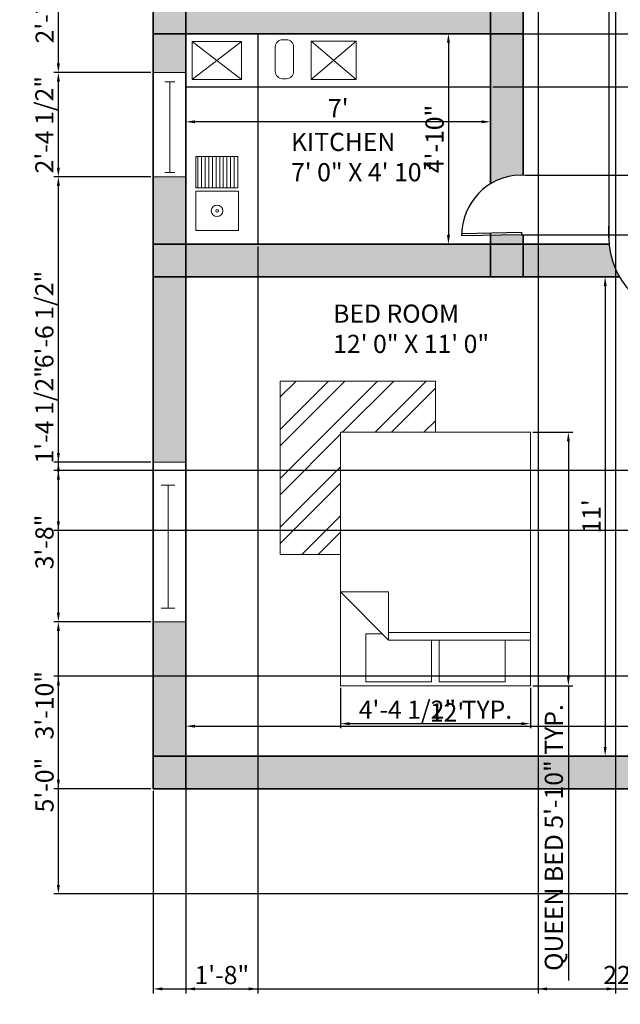
# Model space of a CAD drawing. Units: millimetres. Extents: x 2803 to 3393, y 965 to 1464.
# Tile 1 of 6: x 2803 to 2968, y 965 to 1236. Entities that reach past the tile are written whole.
import ezdxf

# ---------------------------------------------------------------- set-up
doc = ezdxf.new("R2010")
doc.units = ezdxf.units.MM
for name, color, linetype, lineweight in [('A-ANNO-DIMS', 150, 'Continuous', 18), ('A-AREA-IDEN', 200, 'Continuous', 25), ('A-FLOR-CASE', 70, 'Continuous', 25), ('A-FLOR-FIXT', 70, 'Continuous', 18), ('A-FLOR-FIXT-PATT', 70, 'Continuous', 13), ('A-FLOR-PATT', 3, 'Continuous', 13), ('A-WALL-PATT', 2, 'Continuous', 13), ('doors', 10, 'Continuous', 25), ('furniture', 70, 'Continuous', 18), ('walls', 2, 'Continuous', 35), ('windows', 30, 'Continuous', 20)]:
    doc.layers.add(name, color=color, linetype=linetype, lineweight=lineweight)
doc.styles.get("Standard").update_dxf_attribs({"font": 'arial.ttf'})
doc.dimstyles.new('ISO-25', dxfattribs={"dimtxt": 5, "dimasz": 2.5, "dimexe": 1.25, "dimexo": 0.625, "dimtad": 1, "dimdec": 0, "dimlunit": 3, "dimtxsty": 'Standard', "dimcen": 2.5, "dimadec": 0, "dimazin": 0, "dimtfac": 1, "dimtdec": 0, "dimtmove": 0, "dimatfit": 3, "dimfxl": 1, "dimarcsym": 0})

# ---------------------------------------------------------------- blocks, each defined once
blk = doc.blocks.new('*U2')
for p, q in [((0, 0), (0, -6)), ((40, 0), (40, -6))]:
    blk.add_line(p, q)
blk.add_lwpolyline([(0, 0), (0, 40), (1.75, 40), (1.75, 0)], close=True)
blk.add_arc((0, 0), 40, 0, 90)
blk = doc.blocks.new('*U6')
for p, q in [((0, 4), (0, 0)), ((36, 4), (36, 0)), ((0, 2), (36, 2))]:
    blk.add_line(p, q)
blk = doc.blocks.new('Bed - Queen')
for p, q in [((0, -80.00003), (0, 0)), ((0, 0), (59.99999, 0)), ((59.99999, 0), (59.99999, -80.00003)), ((7.99999, -1.2), (28.79998, -1.2)), ((7.99999, -14.4), (7.99999, -1.2)), ((28.79998, -1.2), (28.79998, -14.4)), ((31.19999, -1.2), (51.99999, -1.2)), ((31.19999, -14.4), (31.19999, -1.2)), ((51.99999, -1.2), (51.99999, -16.4)), ((0, -14.4), (44.8, -14.4)), ((59.99999, -29.6), (44.8, -14.4)), ((44.8, -14.4), (44.8, -29.6)), ((44.8, -16.8), (0, -16.8)), ((51.99999, -16.4), (46.79936, -16.4)), ((44.8, -29.6), (59.99999, -29.6)), ((59.99999, -80.00003), (0, -80.00003))]:
    blk.add_line(p, q)
blk = doc.blocks.new('*D22')
at = {"layer": 'A-ANNO-DIMS', "color": 0, "lineweight": -2, "transparency": 16777216}
for p, q in [((2848.68, 1208.91), (2848.68, 1209.54)), ((2930.18, 1208.29), (2851.18, 1208.29)), ((2932.68, 1208.91), (2932.68, 1209.54))]:
    blk.add_line(p, q, dxfattribs=at)
at = {"layer": 'A-ANNO-DIMS', "color": 0, "transparency": 16777216}
for points in [[(2851.18, 1208.7), (2851.18, 1207.87), (2848.68, 1208.29)], [(2930.18, 1208.7), (2930.18, 1207.87), (2932.68, 1208.29)]]:
    blk.add_solid(points, dxfattribs=at)
at = {"layer": 'Defpoints', "color": 0, "transparency": 16777216}
for p in [(2848.68, 1208.29), (2848.68, 1208.29), (2932.68, 1208.29)]:
    blk.add_point(p, dxfattribs=at)
at = {"layer": 'A-ANNO-DIMS', "color": 0, "transparency": 16777216, "insert": (2890.68, 1211.41), "char_height": 5, "attachment_point": 5}
blk.add_mtext("7'", dxfattribs=at)
blk = doc.blocks.new('*D23')
at = {"layer": 'A-ANNO-DIMS', "color": 0, "lineweight": -2, "transparency": 16777216}
for p, q in [((2921.69, 1232.56), (2922.31, 1232.56)), ((2921.06, 1230.06), (2921.06, 1177.06)), ((2921.69, 1174.56), (2922.31, 1174.56))]:
    blk.add_line(p, q, dxfattribs=at)
at = {"layer": 'A-ANNO-DIMS', "color": 0, "transparency": 16777216}
for points in [[(2920.65, 1230.06), (2921.48, 1230.06), (2921.06, 1232.56)], [(2920.65, 1177.06), (2921.48, 1177.06), (2921.06, 1174.56)]]:
    blk.add_solid(points, dxfattribs=at)
at = {"layer": 'Defpoints', "color": 0, "transparency": 16777216}
for p in [(2921.06, 1232.56), (2921.06, 1174.56), (2921.06, 1174.56)]:
    blk.add_point(p, dxfattribs=at)
at = {"layer": 'A-ANNO-DIMS', "color": 0, "transparency": 16777216, "insert": (2917.88, 1203.56), "char_height": 5, "attachment_point": 5, "rotation": 90}
blk.add_mtext('4\'-10"', dxfattribs=at)
blk = doc.blocks.new('*D24')
at = {"layer": 'A-ANNO-DIMS', "color": 0, "lineweight": -2, "transparency": 16777216}
for p, q in [((2959.49, 1165.56), (2965.51, 1165.56)), ((2964.26, 1163.06), (2964.26, 1036.06)), ((2959.49, 1033.56), (2965.51, 1033.56))]:
    blk.add_line(p, q, dxfattribs=at)
at = {"layer": 'A-ANNO-DIMS', "color": 0, "transparency": 16777216}
for points in [[(2963.85, 1163.06), (2964.68, 1163.06), (2964.26, 1165.56)], [(2963.85, 1036.06), (2964.68, 1036.06), (2964.26, 1033.56)]]:
    blk.add_solid(points, dxfattribs=at)
at = {"layer": 'Defpoints', "color": 0, "transparency": 16777216}
for p in [(2958.86, 1165.56), (2958.86, 1033.56), (2964.26, 1033.56)]:
    blk.add_point(p, dxfattribs=at)
at = {"layer": 'A-ANNO-DIMS', "color": 0, "transparency": 16777216, "insert": (2961.13, 1099.56), "char_height": 5, "attachment_point": 5, "rotation": 90}
blk.add_mtext("11'", dxfattribs=at)
blk = doc.blocks.new('*D25')
at = {"layer": 'A-ANNO-DIMS', "color": 0, "lineweight": -2, "transparency": 16777216}
for p, q in [((2848.68, 1045.62), (2848.68, 1040.53)), ((2992.68, 1045.62), (2992.68, 1040.53)), ((2851.18, 1041.78), (2990.18, 1041.78))]:
    blk.add_line(p, q, dxfattribs=at)
at = {"layer": 'A-ANNO-DIMS', "color": 0, "transparency": 16777216}
for points in [[(2851.18, 1042.2), (2851.18, 1041.37), (2848.68, 1041.78)], [(2990.18, 1042.2), (2990.18, 1041.37), (2992.68, 1041.78)]]:
    blk.add_solid(points, dxfattribs=at)
at = {"layer": 'Defpoints', "color": 0, "transparency": 16777216}
for p in [(2848.68, 1046.25), (2992.68, 1046.25), (2992.68, 1041.78)]:
    blk.add_point(p, dxfattribs=at)
at = {"layer": 'A-ANNO-DIMS', "color": 0, "transparency": 16777216, "insert": (2920.68, 1044.92), "char_height": 5, "attachment_point": 5}
blk.add_mtext("12'", dxfattribs=at)
blk = doc.blocks.new('*D29')
at = {"layer": 'A-ANNO-DIMS', "color": 0, "lineweight": -2, "transparency": 16777216}
for p, q in [((2944.28, 1122.74), (2955.37, 1122.74)), ((2954.12, 1120.24), (2954.12, 1055.44)), ((2944.28, 1052.94), (2955.37, 1052.94)), ((2954.12, 1052.94), (2954.12, 971.75))]:
    blk.add_line(p, q, dxfattribs=at)
at = {"layer": 'A-ANNO-DIMS', "color": 0, "transparency": 16777216}
for points in [[(2953.71, 1120.24), (2954.54, 1120.24), (2954.12, 1122.74)], [(2953.71, 1055.44), (2954.54, 1055.44), (2954.12, 1052.94)]]:
    blk.add_solid(points, dxfattribs=at)
at = {"layer": 'Defpoints', "color": 0, "transparency": 16777216}
for p in [(2943.65, 1122.74), (2943.65, 1052.94), (2954.12, 1052.94)]:
    blk.add_point(p, dxfattribs=at)
at = {"layer": 'A-ANNO-DIMS', "color": 0, "transparency": 16777216, "insert": (2950.76, 1011.1), "char_height": 5, "attachment_point": 5, "rotation": 90}
blk.add_mtext('QUEEN BED 5\'-10" TYP.', dxfattribs=at)
blk = doc.blocks.new('*D30')
at = {"layer": 'A-ANNO-DIMS', "color": 0, "lineweight": -2, "transparency": 16777216}
for p, q in [((2891.3, 1052.31), (2891.3, 1041.22)), ((2943.65, 1052.31), (2943.65, 1041.22)), ((2941.15, 1042.47), (2893.8, 1042.47))]:
    blk.add_line(p, q, dxfattribs=at)
at = {"layer": 'A-ANNO-DIMS', "color": 0, "transparency": 16777216}
for points in [[(2893.8, 1042.88), (2893.8, 1042.05), (2891.3, 1042.47)], [(2941.15, 1042.88), (2941.15, 1042.05), (2943.65, 1042.47)]]:
    blk.add_solid(points, dxfattribs=at)
at = {"layer": 'Defpoints', "color": 0, "transparency": 16777216}
for p in [(2891.3, 1052.94), (2943.65, 1052.94), (2891.3, 1042.47)]:
    blk.add_point(p, dxfattribs=at)
at = {"layer": 'A-ANNO-DIMS', "color": 0, "transparency": 16777216, "insert": (2917.48, 1045.68), "char_height": 5, "attachment_point": 5}
blk.add_mtext('4\'-4 1/2" TYP.', dxfattribs=at)
blk = doc.blocks.new('*D39')
at = {"layer": 'A-ANNO-DIMS', "color": 0, "lineweight": -2, "transparency": 16777216}
for p, q in [((2839.68, 1023.94), (2839.68, 968.15)), ((3362.68, 994.94), (3362.68, 968.15)), ((2842.18, 969.4), (3360.18, 969.4))]:
    blk.add_line(p, q, dxfattribs=at)
at = {"layer": 'A-ANNO-DIMS', "color": 0, "transparency": 16777216}
for points in [[(2842.18, 969.82), (2842.18, 968.99), (2839.68, 969.4)], [(3360.18, 969.82), (3360.18, 968.99), (3362.68, 969.4)]]:
    blk.add_solid(points, dxfattribs=at)
at = {"layer": 'Defpoints', "color": 0, "transparency": 16777216}
for p in [(2839.68, 1024.56), (3362.68, 995.56), (3362.68, 969.4)]:
    blk.add_point(p, dxfattribs=at)
at = {"layer": 'A-ANNO-DIMS', "color": 0, "transparency": 16777216, "insert": (3101.18, 972.58), "char_height": 5, "attachment_point": 5}
blk.add_mtext('43\'-7"', dxfattribs=at)
blk = doc.blocks.new('*D42')
at = {"layer": 'A-ANNO-DIMS', "color": 0, "lineweight": -2, "transparency": 16777216}
for p, q in [((3209.06, 1055.56), (2812.27, 1055.56)), ((2813.52, 998.06), (2813.52, 1053.06)), ((3209.06, 995.56), (2812.27, 995.56))]:
    blk.add_line(p, q, dxfattribs=at)
at = {"layer": 'A-ANNO-DIMS', "color": 0, "transparency": 16777216}
for points in [[(2813.11, 1053.06), (2813.94, 1053.06), (2813.52, 1055.56)], [(2813.11, 998.06), (2813.94, 998.06), (2813.52, 995.56)]]:
    blk.add_solid(points, dxfattribs=at)
at = {"layer": 'Defpoints', "color": 0, "transparency": 16777216}
for p in [(2813.52, 1055.56), (3209.68, 1055.56), (3209.68, 995.56)]:
    blk.add_point(p, dxfattribs=at)
at = {"layer": 'A-ANNO-DIMS', "color": 0, "transparency": 16777216, "insert": (2810.35, 1025.56), "char_height": 5, "attachment_point": 5, "rotation": 90}
blk.add_mtext('5\'-0"', dxfattribs=at)
blk = doc.blocks.new('*D48')
at = {"layer": 'A-ANNO-DIMS', "color": 0, "lineweight": -2, "transparency": 16777216}
for p, q in [((2839.68, 1023.94), (2839.68, 968.15)), ((3106.68, 1023.94), (3106.68, 968.15)), ((2842.18, 969.4), (3104.18, 969.4))]:
    blk.add_line(p, q, dxfattribs=at)
at = {"layer": 'A-ANNO-DIMS', "color": 0, "transparency": 16777216}
for points in [[(2842.18, 969.82), (2842.18, 968.99), (2839.68, 969.4)], [(3104.18, 969.82), (3104.18, 968.99), (3106.68, 969.4)]]:
    blk.add_solid(points, dxfattribs=at)
at = {"layer": 'Defpoints', "color": 0, "transparency": 16777216}
for p in [(2839.68, 1024.56), (3106.68, 1024.56), (3106.68, 969.4)]:
    blk.add_point(p, dxfattribs=at)
at = {"layer": 'A-ANNO-DIMS', "color": 0, "transparency": 16777216, "insert": (2973.18, 972.58), "char_height": 5, "attachment_point": 5}
blk.add_mtext('22\'-3"', dxfattribs=at)
blk = doc.blocks.new('*D54')
at = {"layer": 'A-ANNO-DIMS', "color": 0, "lineweight": -2, "transparency": 16777216}
for p, q in [((2839.06, 1070.54), (2812.27, 1070.54)), ((2813.52, 1027.06), (2813.52, 1068.04)), ((2839.06, 1024.56), (2812.27, 1024.56))]:
    blk.add_line(p, q, dxfattribs=at)
at = {"layer": 'A-ANNO-DIMS', "color": 0, "transparency": 16777216}
for points in [[(2813.11, 1068.04), (2813.94, 1068.04), (2813.52, 1070.54)], [(2813.11, 1027.06), (2813.94, 1027.06), (2813.52, 1024.56)]]:
    blk.add_solid(points, dxfattribs=at)
at = {"layer": 'Defpoints', "color": 0, "transparency": 16777216}
for p in [(2813.52, 1070.54), (2839.68, 1070.54), (2839.68, 1024.56)]:
    blk.add_point(p, dxfattribs=at)
at = {"layer": 'A-ANNO-DIMS', "color": 0, "transparency": 16777216, "insert": (2810.34, 1047.55), "char_height": 5, "attachment_point": 5, "rotation": 90}
blk.add_mtext('3\'-10"', dxfattribs=at)
blk = doc.blocks.new('*D55')
at = {"layer": 'A-ANNO-DIMS', "color": 0, "lineweight": -2, "transparency": 16777216}
for p, q in [((2839.06, 1114.52), (2812.27, 1114.52)), ((2813.52, 1073.04), (2813.52, 1112.02)), ((2839.06, 1070.54), (2812.27, 1070.54))]:
    blk.add_line(p, q, dxfattribs=at)
at = {"layer": 'A-ANNO-DIMS', "color": 0, "transparency": 16777216}
for points in [[(2813.11, 1112.02), (2813.94, 1112.02), (2813.52, 1114.52)], [(2813.11, 1073.04), (2813.94, 1073.04), (2813.52, 1070.54)]]:
    blk.add_solid(points, dxfattribs=at)
at = {"layer": 'Defpoints', "color": 0, "transparency": 16777216}
for p in [(2813.52, 1114.52), (2839.68, 1114.52), (2839.68, 1070.54)]:
    blk.add_point(p, dxfattribs=at)
at = {"layer": 'A-ANNO-DIMS', "color": 0, "transparency": 16777216, "insert": (2810.34, 1092.53), "char_height": 5, "attachment_point": 5, "rotation": 90}
blk.add_mtext('3\'-8"', dxfattribs=at)
blk = doc.blocks.new('*D56')
at = {"layer": 'A-ANNO-DIMS', "color": 0, "lineweight": -2, "transparency": 16777216}
for p, q in [((2839.06, 1193.13), (2812.27, 1193.13)), ((2813.52, 1117.02), (2813.52, 1190.63)), ((2839.06, 1114.52), (2812.27, 1114.52))]:
    blk.add_line(p, q, dxfattribs=at)
at = {"layer": 'A-ANNO-DIMS', "color": 0, "transparency": 16777216}
for points in [[(2813.11, 1190.63), (2813.94, 1190.63), (2813.52, 1193.13)], [(2813.11, 1117.02), (2813.94, 1117.02), (2813.52, 1114.52)]]:
    blk.add_solid(points, dxfattribs=at)
at = {"layer": 'Defpoints', "color": 0, "transparency": 16777216}
for p in [(2813.52, 1193.13), (2839.68, 1193.13), (2839.68, 1114.52)]:
    blk.add_point(p, dxfattribs=at)
at = {"layer": 'A-ANNO-DIMS', "color": 0, "transparency": 16777216, "insert": (2810.31, 1153.82), "char_height": 5, "attachment_point": 5, "rotation": 90}
blk.add_mtext('6\'-6 1/2"', dxfattribs=at)
blk = doc.blocks.new('*D57')
at = {"layer": 'A-ANNO-DIMS', "color": 0, "lineweight": -2, "transparency": 16777216}
for p, q in [((2839.06, 1221.86), (2812.27, 1221.86)), ((2813.52, 1195.63), (2813.52, 1219.36)), ((2839.06, 1193.13), (2812.27, 1193.13))]:
    blk.add_line(p, q, dxfattribs=at)
at = {"layer": 'A-ANNO-DIMS', "color": 0, "transparency": 16777216}
for points in [[(2813.11, 1219.36), (2813.94, 1219.36), (2813.52, 1221.86)], [(2813.11, 1195.63), (2813.94, 1195.63), (2813.52, 1193.13)]]:
    blk.add_solid(points, dxfattribs=at)
at = {"layer": 'Defpoints', "color": 0, "transparency": 16777216}
for p in [(2813.52, 1221.86), (2839.68, 1221.86), (2839.68, 1193.13)]:
    blk.add_point(p, dxfattribs=at)
at = {"layer": 'A-ANNO-DIMS', "color": 0, "transparency": 16777216, "insert": (2810.31, 1207.49), "char_height": 5, "attachment_point": 5, "rotation": 90}
blk.add_mtext('2\'-4 1/2"', dxfattribs=at)
blk = doc.blocks.new('*D58')
at = {"layer": 'A-ANNO-DIMS', "color": 0, "lineweight": -2, "transparency": 16777216}
for p, q in [((2839.06, 1252.94), (2812.27, 1252.94)), ((2813.52, 1224.36), (2813.52, 1250.44)), ((2839.06, 1221.86), (2812.27, 1221.86))]:
    blk.add_line(p, q, dxfattribs=at)
at = {"layer": 'A-ANNO-DIMS', "color": 0, "transparency": 16777216}
for points in [[(2813.11, 1250.44), (2813.94, 1250.44), (2813.52, 1252.94)], [(2813.11, 1224.36), (2813.94, 1224.36), (2813.52, 1221.86)]]:
    blk.add_solid(points, dxfattribs=at)
at = {"layer": 'Defpoints', "color": 0, "transparency": 16777216}
for p in [(2813.52, 1252.94), (2839.68, 1252.94), (2839.68, 1221.86)]:
    blk.add_point(p, dxfattribs=at)
at = {"layer": 'A-ANNO-DIMS', "color": 0, "transparency": 16777216, "insert": (2810.39, 1237.4), "char_height": 5, "attachment_point": 5, "rotation": 90}
blk.add_mtext('2\'-7"', dxfattribs=at)
blk = doc.blocks.new('*D67')
at = {"layer": 'A-ANNO-DIMS', "color": 0, "lineweight": -2, "transparency": 16777216}
for p, q in [((2945.75, 1288.94), (2945.75, 968.15)), ((2967.14, 1288.94), (2967.14, 968.15)), ((2948.25, 969.4), (2964.64, 969.4)), ((2967.14, 969.4), (2995.36, 969.4))]:
    blk.add_line(p, q, dxfattribs=at)
at = {"layer": 'A-ANNO-DIMS', "color": 0, "transparency": 16777216}
for points in [[(2948.25, 969.82), (2948.25, 968.99), (2945.75, 969.4)], [(2964.64, 969.82), (2964.64, 968.99), (2967.14, 969.4)]]:
    blk.add_solid(points, dxfattribs=at)
at = {"layer": 'Defpoints', "color": 0, "transparency": 16777216}
for p in [(2945.75, 1289.56), (2967.14, 1289.56), (2967.14, 969.4)]:
    blk.add_point(p, dxfattribs=at)
at = {"layer": 'A-ANNO-DIMS', "color": 0, "transparency": 16777216, "insert": (2982.5, 972.61), "char_height": 5, "attachment_point": 5}
blk.add_mtext('1\'-9 1/2"', dxfattribs=at)
blk = doc.blocks.new('*D69')
at = {"layer": 'A-ANNO-DIMS', "color": 0, "lineweight": -2, "transparency": 16777216}
for p, q in [((3388.84, 1193.62), (3388.84, 1221.84)), ((2942.31, 1193.62), (3390.09, 1193.62)), ((3388.84, 1179.64), (3388.84, 1191.12)), ((2942.31, 1177.14), (3390.09, 1177.14))]:
    blk.add_line(p, q, dxfattribs=at)
at = {"layer": 'A-ANNO-DIMS', "color": 0, "transparency": 16777216}
for points in [[(3388.43, 1191.12), (3389.26, 1191.12), (3388.84, 1193.62)], [(3388.43, 1179.64), (3389.26, 1179.64), (3388.84, 1177.14)]]:
    blk.add_solid(points, dxfattribs=at)
at = {"layer": 'Defpoints', "color": 0, "transparency": 16777216}
for p in [(2941.68, 1193.62), (3388.84, 1193.62), (2941.68, 1177.14)]:
    blk.add_point(p, dxfattribs=at)
at = {"layer": 'A-ANNO-DIMS', "color": 0, "transparency": 16777216, "insert": (3385.63, 1208.98), "char_height": 5, "attachment_point": 5, "rotation": 90}
blk.add_mtext('1\'-4 1/2"', dxfattribs=at)
blk = doc.blocks.new('*D70')
at = {"layer": 'A-ANNO-DIMS', "color": 0, "lineweight": -2, "transparency": 16777216}
for p, q in [((2965.38, 1175.19), (2965.38, 1454.97)), ((2986.69, 1175.19), (2986.69, 1454.97)), ((2967.88, 1453.72), (2984.19, 1453.72)), ((2986.69, 1453.72), (3014.92, 1453.72))]:
    blk.add_line(p, q, dxfattribs=at)
at = {"layer": 'A-ANNO-DIMS', "color": 0, "transparency": 16777216}
for points in [[(2967.88, 1454.14), (2967.88, 1453.31), (2965.38, 1453.72)], [(2984.19, 1454.14), (2984.19, 1453.31), (2986.69, 1453.72)]]:
    blk.add_solid(points, dxfattribs=at)
at = {"layer": 'Defpoints', "color": 0, "transparency": 16777216}
for p in [(2986.69, 1453.72), (2965.38, 1174.56), (2986.69, 1174.56)]:
    blk.add_point(p, dxfattribs=at)
at = {"layer": 'A-ANNO-DIMS', "color": 0, "transparency": 16777216, "insert": (3002.06, 1456.93), "char_height": 5, "attachment_point": 5}
blk.add_mtext('1\'-9 1/2"', dxfattribs=at)
blk = doc.blocks.new('*D71')
at = {"layer": 'A-ANNO-DIMS', "color": 0, "lineweight": -2, "transparency": 16777216}
for p, q in [((2813.52, 1112.21), (2813.52, 1140.43)), ((2992.06, 1112.21), (2812.27, 1112.21)), ((2813.52, 1098.23), (2813.52, 1109.71)), ((2992.06, 1095.73), (2812.27, 1095.73))]:
    blk.add_line(p, q, dxfattribs=at)
at = {"layer": 'A-ANNO-DIMS', "color": 0, "transparency": 16777216}
for points in [[(2813.11, 1109.71), (2813.94, 1109.71), (2813.52, 1112.21)], [(2813.11, 1098.23), (2813.94, 1098.23), (2813.52, 1095.73)]]:
    blk.add_solid(points, dxfattribs=at)
at = {"layer": 'Defpoints', "color": 0, "transparency": 16777216}
for p in [(2813.52, 1112.21), (2992.68, 1112.21), (2992.68, 1095.73)]:
    blk.add_point(p, dxfattribs=at)
at = {"layer": 'A-ANNO-DIMS', "color": 0, "transparency": 16777216, "insert": (2810.31, 1127.57), "char_height": 5, "attachment_point": 5, "rotation": 90}
blk.add_mtext('1\'-4 1/2"', dxfattribs=at)
blk = doc.blocks.new('*D73')
at = {"layer": 'A-ANNO-DIMS', "color": 0, "lineweight": -2, "transparency": 16777216}
for p, q in [((2848.68, 1217.26), (2848.68, 968.15)), ((2868.49, 1173.94), (2868.49, 968.15)), ((2851.18, 969.4), (2865.99, 969.4))]:
    blk.add_line(p, q, dxfattribs=at)
at = {"layer": 'A-ANNO-DIMS', "color": 0, "transparency": 16777216}
for points in [[(2851.18, 969.82), (2851.18, 968.99), (2848.68, 969.4)], [(2865.99, 969.82), (2865.99, 968.99), (2868.49, 969.4)]]:
    blk.add_solid(points, dxfattribs=at)
at = {"layer": 'Defpoints', "color": 0, "transparency": 16777216}
for p in [(2848.68, 1217.89), (2868.49, 1174.56), (2868.49, 969.4)]:
    blk.add_point(p, dxfattribs=at)
at = {"layer": 'A-ANNO-DIMS', "color": 0, "transparency": 16777216, "insert": (2858.59, 972.58), "char_height": 5, "attachment_point": 5}
blk.add_mtext('1\'-8"', dxfattribs=at)
blk = doc.blocks.new('*D74')
at = {"layer": 'A-ANNO-DIMS', "color": 0, "lineweight": -2, "transparency": 16777216}
for p, q in [((3388.84, 1232.56), (3388.84, 1260.78)), ((2869.11, 1232.56), (3390.09, 1232.56)), ((3388.84, 1220.39), (3388.84, 1230.06)), ((2933.31, 1217.89), (3390.09, 1217.89))]:
    blk.add_line(p, q, dxfattribs=at)
at = {"layer": 'A-ANNO-DIMS', "color": 0, "transparency": 16777216}
for points in [[(3388.43, 1230.06), (3389.26, 1230.06), (3388.84, 1232.56)], [(3388.43, 1220.39), (3389.26, 1220.39), (3388.84, 1217.89)]]:
    blk.add_solid(points, dxfattribs=at)
at = {"layer": 'Defpoints', "color": 0, "transparency": 16777216}
for p in [(2868.49, 1232.56), (3388.84, 1232.56), (2932.68, 1217.89)]:
    blk.add_point(p, dxfattribs=at)
at = {"layer": 'A-ANNO-DIMS', "color": 0, "transparency": 16777216, "insert": (3385.63, 1247.92), "char_height": 5, "attachment_point": 5, "rotation": 90}
blk.add_mtext('1\'-2 1/2"', dxfattribs=at)

msp = doc.modelspace()

# ---------------------------------------------------------------- hatches: boundary and pattern name
at = {"layer": 'A-FLOR-FIXT-PATT'}
h = msp.add_hatch(dxfattribs=at)
h.set_pattern_fill('ANSI31', color=256, scale=0.3149606, angle=45, style=0)
h.paths.add_polyline_path([(2851.43, 1190.1), (2862.97, 1190.1), (2862.97, 1198.74), (2851.43, 1198.74)])
at = {"layer": 'A-FLOR-PATT'}
h = msp.add_hatch(dxfattribs=at)
h.set_pattern_fill('ANSI32', color=256)
h.paths.add_polyline_path([(2935.82, 1362.49), (2919.19, 1362.49), (2919.19, 1328.83), (2893.01, 1328.83), (2893.01, 1314.7), (2935.82, 1314.7)])
h.paths.add_polyline_path([(2891.3, 1122.74), (2917.48, 1122.74), (2917.48, 1136.87), (2874.67, 1136.87), (2874.67, 1089.08), (2891.3, 1089.08)])
at = {"layer": 'A-WALL-PATT'}
h = msp.add_hatch(color=256, dxfattribs=at)
h.dxf.hatch_style = 1
h.paths.add_polyline_path([(2968.68, 1427.56), (2919.98, 1427.56), (2919.98, 1418.56), (2968.68, 1418.56)])
h.paths.add_polyline_path([(2977.68, 1427.56), (2968.68, 1427.56), (2968.68, 1418.56), (2977.68, 1418.56)])
h.paths.add_polyline_path([(2977.68, 1418.56), (2968.68, 1418.56), (2968.68, 1298.56), (2977.68, 1298.56)])
h.paths.add_polyline_path([(3021.74, 1427.56), (2977.68, 1427.56), (2977.68, 1418.56), (3021.74, 1418.56)])
h.paths.add_polyline_path([(2881.7, 1427.56), (2848.68, 1427.56), (2848.68, 1418.56), (2881.7, 1418.56)])
h.paths.add_polyline_path([(2848.68, 1427.56), (2839.68, 1427.56), (2839.68, 1418.56), (2848.68, 1418.56)])
h.paths.add_polyline_path([(2848.68, 1418.56), (2839.68, 1418.56), (2839.68, 1298.56), (2848.68, 1298.56)])
h.paths.add_polyline_path([(2932.68, 1298.56), (2848.68, 1298.56), (2848.68, 1289.56), (2932.68, 1289.56)])
h.paths.add_polyline_path([(2848.68, 1298.56), (2839.68, 1298.56), (2839.68, 1289.56), (2848.68, 1289.56)])
h.paths.add_polyline_path([(2848.68, 1289.56), (2839.68, 1289.56), (2839.68, 1280.88), (2848.68, 1280.88)])
h.paths.add_polyline_path([(2848.68, 1252.94), (2839.68, 1252.94), (2839.68, 1241.56), (2848.68, 1241.56)])
h.paths.add_polyline_path([(2848.68, 1241.56), (2839.68, 1241.56), (2839.68, 1232.56), (2848.68, 1232.56)])
h.paths.add_polyline_path([(2932.68, 1241.56), (2848.68, 1241.56), (2848.68, 1232.56), (2932.68, 1232.56)])
h.paths.add_polyline_path([(2941.68, 1241.56), (2932.68, 1241.56), (2932.68, 1232.56), (2941.68, 1232.56)])
h.paths.add_polyline_path([(2941.68, 1289.56), (2932.68, 1289.56), (2932.68, 1257.22, -0.114666), (2939.92, 1259.03), (2941.68, 1259.07)])
h.paths.add_polyline_path([(2941.68, 1298.56), (2932.68, 1298.56), (2932.68, 1289.56), (2941.68, 1289.56)])
h.paths.add_polyline_path([(2947.42, 1298.56), (2941.68, 1298.56), (2941.68, 1289.56), (2945.75, 1289.56), (2945.75, 1290.29, -0.099582)])
h.paths.add_polyline_path([(2977.68, 1298.56), (2968.68, 1298.56), (2968.68, 1289.56), (2977.68, 1289.56)])
h.paths.add_polyline_path([(3018.47, 1298.56), (2977.68, 1298.56), (2977.68, 1289.56), (3018.47, 1289.56)])
h.paths.add_polyline_path([(3097.68, 1298.56), (3067.31, 1298.56), (3067.31, 1289.56), (3097.68, 1289.56)])
h.paths.add_polyline_path([(3106.68, 1298.56), (3097.68, 1298.56), (3097.68, 1289.56), (3106.68, 1289.56)])
h.paths.add_polyline_path([(3200.68, 1298.56), (3106.68, 1298.56), (3106.68, 1289.56), (3200.68, 1289.56)])
h.paths.add_polyline_path([(3209.68, 1298.56), (3200.68, 1298.56), (3200.68, 1289.56), (3209.68, 1289.56)])
h.paths.add_polyline_path([(3209.68, 1289.56), (3200.68, 1289.56), (3200.68, 1270.22), (3209.68, 1270.22)])
h.paths.add_polyline_path([(3106.68, 1418.56), (3097.68, 1418.56), (3097.68, 1298.56), (3106.68, 1298.56)])
h.paths.add_polyline_path([(3106.68, 1427.56), (3097.68, 1427.56), (3097.68, 1418.56), (3106.68, 1418.56)])
h.paths.add_polyline_path([(3097.68, 1427.56), (3058.94, 1427.56), (3058.94, 1418.56), (3097.68, 1418.56)])
h.paths.add_polyline_path([(3353.68, 1427.56), (3106.68, 1427.56), (3106.68, 1418.56), (3353.68, 1418.56)])
h.paths.add_polyline_path([(3362.68, 1427.56), (3353.68, 1427.56), (3353.68, 1418.56), (3362.68, 1418.56)])
h.paths.add_polyline_path([(3362.68, 1418.56), (3353.68, 1418.56), (3353.68, 1064.56), (3362.68, 1064.56)])
h.paths.add_polyline_path([(3362.68, 1064.56), (3353.68, 1064.56), (3353.68, 1055.56), (3362.68, 1055.56)])
h.paths.add_polyline_path([(3362.68, 1055.56), (3353.68, 1055.56), (3353.68, 995.56), (3362.68, 995.56)])
h.paths.add_polyline_path([(3353.68, 1064.56), (3209.68, 1064.56), (3209.68, 1055.56), (3353.68, 1055.56)])
h.paths.add_polyline_path([(3200.68, 1064.56), (3106.68, 1064.56), (3106.68, 1055.56), (3200.68, 1055.56)])
h.paths.add_polyline_path([(3209.68, 1064.56), (3200.68, 1064.56), (3200.68, 1055.56), (3209.68, 1055.56)])
h.paths.add_polyline_path([(3209.68, 1229.61), (3200.68, 1229.61), (3200.68, 1064.56), (3209.68, 1064.56)])
h.paths.add_polyline_path([(3106.68, 1117.56), (3097.68, 1117.56), (3097.68, 1064.56), (3106.68, 1064.56)])
h.paths.add_polyline_path([(3106.68, 1126.56), (3097.68, 1126.56), (3097.68, 1117.56), (3106.68, 1117.56)])
h.paths.add_polyline_path([(3097.68, 1126.56), (3001.68, 1126.56), (3001.68, 1117.56), (3097.68, 1117.56)])
h.paths.add_polyline_path([(3001.68, 1165.56), (2992.68, 1165.56), (2992.68, 1126.56), (3001.68, 1126.56)])
h.paths.add_polyline_path([(3001.68, 1174.56), (2992.68, 1174.56), (2992.68, 1165.56), (3001.68, 1165.56)])
h.paths.add_polyline_path([(2992.68, 1174.56), (2986.69, 1174.56), (2986.69, 1165.56), (2992.68, 1165.56)])
h.paths.add_polyline_path([(3001.68, 1126.56), (2992.68, 1126.56), (2992.68, 1117.56), (3001.68, 1117.56)])
h.paths.add_polyline_path([(3001.68, 1117.56), (2992.68, 1117.56), (2992.68, 1112.21), (2994.15, 1112.23), (3001.68, 1112.37)])
h.paths.add_polyline_path([(3001.68, 1033.56), (2992.68, 1033.56), (2992.68, 1024.56), (3001.68, 1024.56)])
h.paths.add_polyline_path([(3001.68, 1097.58, -0.114732), (2994.45, 1095.76), (2992.68, 1095.73), (2992.68, 1033.56), (3001.68, 1033.56)])
h.paths.add_polyline_path([(3030.4, 1033.56), (3001.68, 1033.56), (3001.68, 1024.56), (3030.4, 1024.56)])
h.paths.add_polyline_path([(3097.68, 1033.56), (3060.2, 1033.56), (3060.2, 1024.56), (3097.68, 1024.56)])
h.paths.add_polyline_path([(3106.68, 1033.56), (3097.68, 1033.56), (3097.68, 1024.56), (3106.68, 1024.56)])
h.paths.add_polyline_path([(3106.68, 1055.56), (3097.68, 1055.56), (3097.68, 1033.56), (3106.68, 1033.56)])
h.paths.add_polyline_path([(3106.68, 1064.56), (3097.68, 1064.56), (3097.68, 1055.56), (3106.68, 1055.56)])
h.paths.add_polyline_path([(2992.68, 1033.56), (2848.68, 1033.56), (2848.68, 1024.56), (2992.68, 1024.56)])
h.paths.add_polyline_path([(2848.68, 1033.56), (2839.68, 1033.56), (2839.68, 1024.56), (2848.68, 1024.56)])
h.paths.add_polyline_path([(2848.68, 1070.54), (2839.68, 1070.54), (2839.68, 1033.56), (2848.68, 1033.56)])
h.paths.add_polyline_path([(2848.68, 1165.56), (2839.68, 1165.56), (2839.68, 1114.52), (2848.68, 1114.52)])
h.paths.add_polyline_path([(2848.68, 1174.56), (2839.68, 1174.56), (2839.68, 1165.56), (2848.68, 1165.56)])
h.paths.add_polyline_path([(2932.68, 1174.56), (2848.68, 1174.56), (2848.68, 1165.56), (2932.68, 1165.56)])
h.paths.add_polyline_path([(2941.68, 1174.56), (2932.68, 1174.56), (2932.68, 1165.56), (2941.68, 1165.56)])
h.paths.add_polyline_path([(2965.38, 1174.56), (2941.68, 1174.56), (2941.68, 1165.56), (2968.2, 1165.56, -0.111634)])
h.paths.add_polyline_path([(2848.68, 1193.13), (2839.68, 1193.13), (2839.68, 1174.56), (2848.68, 1174.56)])
h.paths.add_polyline_path([(2848.68, 1232.56), (2839.68, 1232.56), (2839.68, 1221.86), (2848.68, 1221.86)])
h.paths.add_polyline_path([(2941.68, 1232.56), (2932.68, 1232.56), (2932.68, 1191.24, -0.132111), (2940.91, 1193.6), (2941.68, 1193.62)])
h.paths.add_polyline_path([(3106.68, 1262.96), (3105.94, 1262.96, -0.099353), (3097.68, 1264.61), (3097.68, 1126.56), (3106.68, 1126.56)])
h = msp.add_hatch(color=256, dxfattribs=at)
h.dxf.hatch_style = 1
h.paths.add_polyline_path([(2941.68, 1177.14), (2941.2, 1177.13), (2932.68, 1176.98), (2932.68, 1174.56), (2941.68, 1174.56)])

# ---------------------------------------------------------------- linework, layer by layer
at = {"layer": 'A-FLOR-CASE'}
for p, q in [((2868.49, 1232.56), (2868.49, 1174.56)), ((2848.68, 1217.89), (2932.68, 1217.89))]:
    msp.add_line(p, q, dxfattribs=at)
at = {"layer": 'A-FLOR-FIXT'}
for p, q in [((2850.37, 1230.39), (2863.99, 1219.92)), ((2863.99, 1230.39), (2850.37, 1219.92)), ((2883.25, 1230.46), (2895.62, 1219.94)), ((2895.62, 1230.46), (2883.25, 1219.94))]:
    msp.add_line(p, q, dxfattribs=at)
for points in [[(2850.37, 1230.39), (2863.99, 1230.39), (2863.99, 1219.92), (2850.37, 1219.92)], [(2883.25, 1230.46), (2895.62, 1230.46), (2895.62, 1219.94), (2883.25, 1219.94)], [(2851.43, 1190.1), (2862.97, 1190.1), (2862.97, 1198.74), (2851.43, 1198.74)], [(2851.38, 1178.37), (2863.16, 1178.37), (2863.16, 1189.16), (2851.38, 1189.16)]]:
    msp.add_lwpolyline(points, close=True, dxfattribs=at)
msp.add_lwpolyline([(2875.31, 1230.89), (2876.39, 1230.89, -0.414214), (2878.39, 1228.89), (2878.39, 1222.17, -0.414214), (2876.39, 1220.17), (2875.31, 1220.17, -0.414214), (2873.31, 1222.17), (2873.31, 1228.89, -0.414214)], format="xyb", close=True, dxfattribs=at)
for radius in [1.59, 0.375]:
    msp.add_circle((2857.27, 1183.76), radius, dxfattribs=at)
at = {"layer": 'furniture'}
for p, q in [((2874.67, 1089.08), (2874.67, 1136.87)), ((2874.67, 1136.87), (2917.48, 1136.87)), ((2917.48, 1136.87), (2917.48, 1122.74)), ((2891.3, 1089.08), (2874.67, 1089.08))]:
    msp.add_line(p, q, dxfattribs=at)
at = {"layer": 'walls'}
for p, q in [((2839.68, 1427.56), (2839.68, 1024.56)), ((2848.68, 1427.56), (2848.68, 1024.56)), ((2941.68, 1242.59), (2941.68, 1193.62)), ((2932.68, 1241.56), (2932.68, 1191.24)), ((2839.68, 1232.56), (2941.68, 1232.56)), ((2932.68, 1177.7), (2932.68, 1165.56)), ((2839.68, 1174.56), (2965.38, 1174.56)), ((2941.68, 1177.14), (2941.68, 1165.56)), ((2839.68, 1165.56), (2968.2, 1165.56)), ((2839.68, 1033.56), (3106.68, 1033.56)), ((2839.68, 1024.56), (3106.68, 1024.56))]:
    msp.add_line(p, q, dxfattribs=at)
at = {"layer": 'windows'}
for p, q in [((2848.68, 1221.86), (2839.68, 1221.86)), ((2848.68, 1193.13), (2839.68, 1193.13)), ((2848.68, 1114.52), (2839.68, 1114.52)), ((2848.68, 1070.54), (2839.68, 1070.54))]:
    msp.add_line(p, q, dxfattribs=at)

# ---------------------------------------------------------------- block references
at = {"layer": 'doors'}
for p, xscale, yscale, zscale, rotation in [((2941.2, 1177.13), 0.4118610338034785, 0.4118610338034785, 0.4118610338034785, 91.02414730254725), ((2986.69, 1176.32), 0.534749261424752, 0.534749261424752, 0.534749261424752, 180)]:
    msp.add_blockref('*U2', p, dxfattribs=dict(at, xscale=xscale, yscale=yscale, zscale=zscale, rotation=rotation))
at = {"layer": 'furniture', "xscale": 0.8725478545565646, "yscale": 0.8725478545565646, "zscale": 0.8725478545565646, "rotation": 180}
msp.add_blockref('Bed - Queen', (2943.65, 1052.94), dxfattribs=at)
at = {"layer": 'windows', "rotation": 90}
for p, xscale, yscale, zscale in [((2845.65, 1194.29), 0.6948136988430634, 0.6948136988430634, 0.6948136988430634), ((2845.65, 1074.27), 0.9425308196764994, 0.9425308196764994, 0.9425308196764994)]:
    msp.add_blockref('*U6', p, dxfattribs=dict(at, xscale=xscale, yscale=yscale, zscale=zscale))

# ---------------------------------------------------------------- texts
at = {"layer": 'A-AREA-IDEN', "char_height": 5, "attachment_point": 1}
for s, width, insert in [('KITCHEN \\P7\' 0" X 4\' 10"', 39.4239, (2877.66, 1205.24)), ('BED ROOM \\P12\' 0" X 11\' 0"', 61.4615, (2889.28, 1157.94))]:
    msp.add_mtext_dynamic_manual_height_columns(s, width=width, gutter_width=12.5, heights=[0], dxfattribs=dict(at, insert=insert))

# ---------------------------------------------------------------- dimensions: what is measured, and where the dimension line sits
at = {"layer": 'A-ANNO-DIMS'}
for base, p1, p2, override, picture, middle in [((2986.69, 1453.72), (2965.38, 1174.56), (2986.69, 1174.56), {"dimdec": 1, "dimlfac": 1, "dimrnd": 0, "dimzin": 1, "dimdsep": 46, "dimlunit": 4, "dimfrac": 2}, '*D70', (3002.06, 1456.93)), ((2967.14, 969.4), (2945.75, 1289.56), (2967.14, 1289.56), {"dimdec": 1, "dimlfac": 1, "dimrnd": 0, "dimzin": 1, "dimdsep": 46, "dimlunit": 4, "dimfrac": 2}, '*D67', (2982.5, 972.61)), ((2868.49, 969.4), (2848.68, 1217.89), (2868.49, 1174.56), {"dimdec": 1, "dimlfac": 1, "dimrnd": 0, "dimzin": 1, "dimdsep": 46, "dimlunit": 4, "dimfrac": 2}, '*D73', (2858.59, 972.58)), ((2848.68, 1208.29), (2932.68, 1208.29), (2848.68, 1208.29), {"dimclrd": 0, "dimclre": 0, "dimclrt": 0}, '*D22', (2890.68, 1211.41)), ((2992.68, 1041.78), (2848.68, 1046.25), (2992.68, 1046.25), {"dimclrd": 0, "dimclre": 0, "dimclrt": 0}, '*D25', (2920.68, 1044.92)), ((3362.68, 969.4), (2839.68, 1024.56), (3362.68, 995.56), {"dimdec": 1, "dimlfac": 1, "dimrnd": 0, "dimzin": 1, "dimdsep": 46, "dimlunit": 4, "dimfrac": 2}, '*D39', (3101.18, 972.58)), ((3106.68, 969.4), (2839.68, 1024.56), (3106.68, 1024.56), {"dimdec": 1, "dimlfac": 1, "dimrnd": 0, "dimzin": 1, "dimdsep": 46, "dimlunit": 4, "dimfrac": 2}, '*D48', (2973.18, 972.58))]:
    dim = msp.add_linear_dim(base=base, p1=p1, p2=p2, dimstyle='ISO-25', override=override, dxfattribs=at)
    dim.commit()
    dim.dimension.update_dxf_attribs({"geometry": picture, "text_midpoint": middle})
for base, p1, p2, override, picture, middle in [((3388.84, 1232.56), (2932.68, 1217.89), (2868.49, 1232.56), {"dimdec": 1, "dimlfac": 1, "dimrnd": 0, "dimzin": 1, "dimdsep": 46, "dimlunit": 4, "dimfrac": 2}, '*D74', (3385.63, 1247.92)), ((2813.52, 1252.94), (2839.68, 1221.86), (2839.68, 1252.94), {"dimdec": 1, "dimlfac": 1, "dimrnd": 0, "dimzin": 1, "dimdsep": 46, "dimlunit": 4, "dimfrac": 2}, '*D58', (2810.39, 1237.4)), ((2921.06, 1174.56), (2921.06, 1232.56), (2921.06, 1174.56), {"dimclrd": 0, "dimclre": 0, "dimclrt": 0}, '*D23', (2917.88, 1203.56)), ((2813.52, 1221.86), (2839.68, 1193.13), (2839.68, 1221.86), {"dimdec": 1, "dimlfac": 1, "dimrnd": 0, "dimzin": 1, "dimdsep": 46, "dimlunit": 4, "dimfrac": 2}, '*D57', (2810.31, 1207.49)), ((3388.84, 1193.62), (2941.68, 1177.14), (2941.68, 1193.62), {"dimdec": 1, "dimlfac": 1, "dimrnd": 0, "dimzin": 1, "dimdsep": 46, "dimlunit": 4, "dimfrac": 2}, '*D69', (3385.63, 1208.98)), ((2813.52, 1193.13), (2839.68, 1114.52), (2839.68, 1193.13), {"dimdec": 1, "dimlfac": 1, "dimrnd": 0, "dimzin": 1, "dimdsep": 46, "dimlunit": 4, "dimfrac": 2}, '*D56', (2810.31, 1153.82)), ((2964.26, 1033.56), (2958.86, 1165.56), (2958.86, 1033.56), {"dimclrd": 0, "dimclre": 0, "dimclrt": 0}, '*D24', (2961.13, 1099.56)), ((2813.52, 1112.21), (2992.68, 1095.73), (2992.68, 1112.21), {"dimdec": 1, "dimlfac": 1, "dimrnd": 0, "dimzin": 1, "dimdsep": 46, "dimlunit": 4, "dimfrac": 2}, '*D71', (2810.31, 1127.57)), ((2813.52, 1114.52), (2839.68, 1070.54), (2839.68, 1114.52), {"dimdec": 1, "dimlfac": 1, "dimrnd": 0, "dimzin": 1, "dimdsep": 46, "dimlunit": 4, "dimfrac": 2}, '*D55', (2810.34, 1092.53)), ((2813.52, 1070.54), (2839.68, 1024.56), (2839.68, 1070.54), {"dimdec": 1, "dimlfac": 1, "dimrnd": 0, "dimzin": 1, "dimdsep": 46, "dimlunit": 4, "dimfrac": 2}, '*D54', (2810.34, 1047.55)), ((2813.52, 1055.56), (3209.68, 995.56), (3209.68, 1055.56), {"dimdec": 1, "dimlfac": 1, "dimrnd": 0, "dimzin": 1, "dimdsep": 46, "dimlunit": 4, "dimfrac": 2}, '*D42', (2810.35, 1025.56))]:
    dim = msp.add_linear_dim(base=base, p1=p1, p2=p2, angle=90, dimstyle='ISO-25', override=override, dxfattribs=at)
    dim.commit()
    dim.dimension.update_dxf_attribs({"geometry": picture, "text_midpoint": middle})
for base, p1, p2, angle, text, picture, middle in [((2954.12, 1052.94), (2943.65, 1122.74), (2943.65, 1052.94), 270, 'QUEEN BED <> TYP.', '*D29', (2950.76, 1011.1)), ((2891.3008, 1042.4671), (2943.6536, 1052.9377), (2891.3008, 1052.9377), 180, '<> TYP.', '*D30', (2917.4772, 1045.6774))]:
    dim = msp.add_linear_dim(base=base, p1=p1, p2=p2, angle=angle, text=text, dimstyle='ISO-25', override={"dimdec": 1, "dimlfac": 1, "dimrnd": 0, "dimzin": 1, "dimdsep": 46, "dimlunit": 4, "dimfrac": 2}, dxfattribs=at)
    dim.commit()
    dim.dimension.update_dxf_attribs({"geometry": picture, "text_midpoint": middle})

doc.saveas('drawing.dxf')
